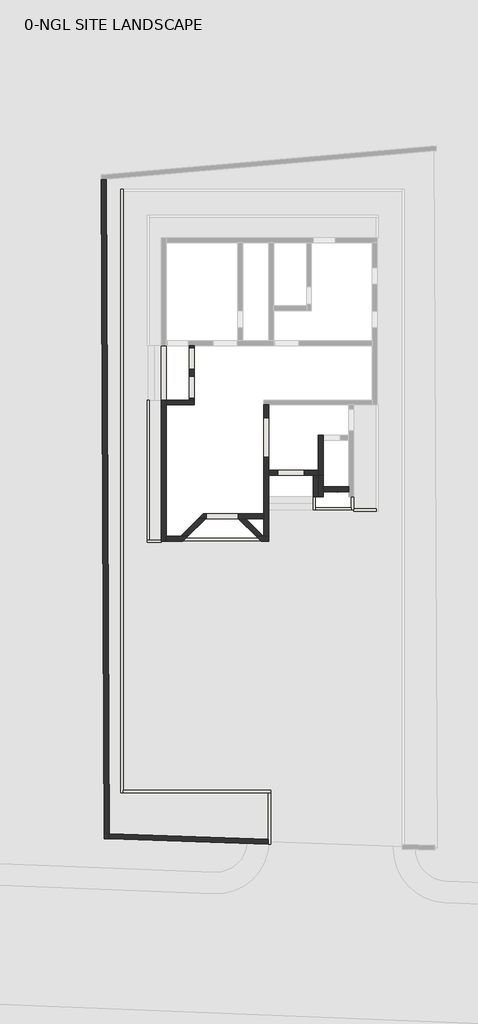
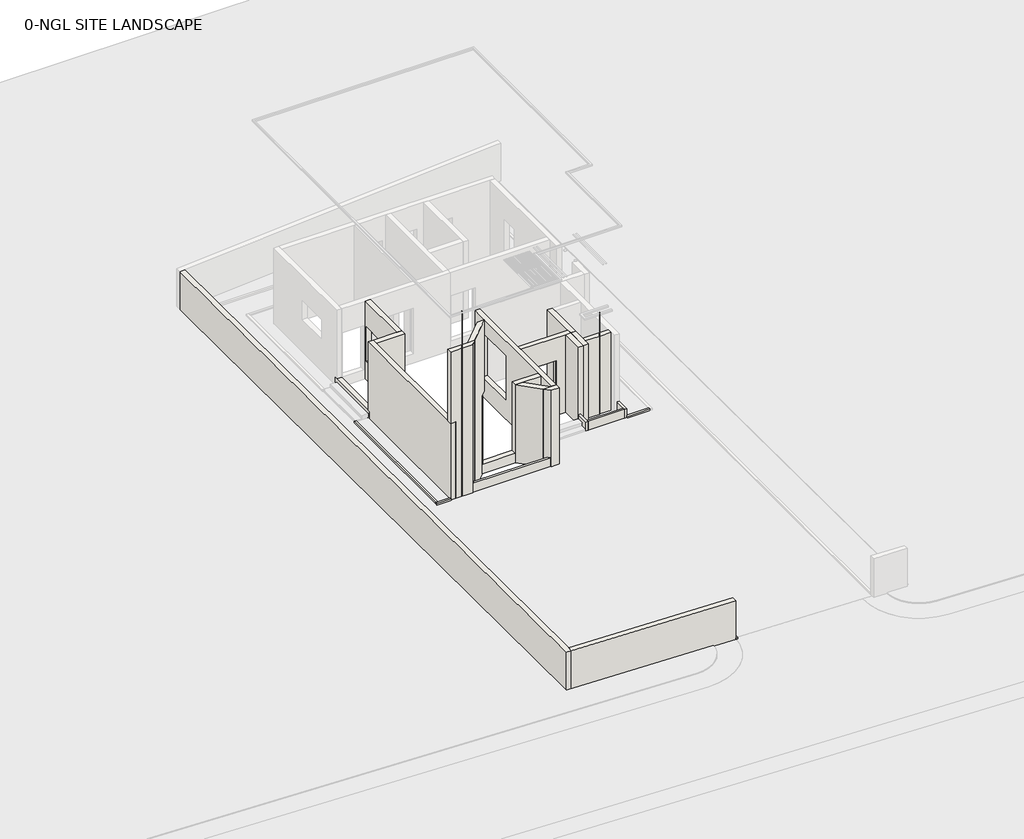
# One storey, part 1 of 2: 27 walls, 2 proxies.
"""IFC4 building model written with IfcOpenShell, lengths in millimetres."""

from ifc_helpers import new_model, si_unit, point, frame, frame_2d, origin, origin_with_axes, place, context, project, spatial, polyline, circle_curve, trimmed, segment, composite_curve, outline, extrude, faceted_brep, element, save
from ifc_brep_helpers import plane_surface, revolved_surface, advanced_brep

model = new_model("IFC4")

# Units and contexts
model_context = context("Model", 3, world=origin())
ifc_project = project(units=[si_unit("LENGTHUNIT", "METRE", prefix="MILLI")], contexts=[model_context])

# Site, building, storey
site = spatial("IfcSite", under=ifc_project)
building = spatial("IfcBuilding", under=site)
storey = spatial("IfcBuildingStorey", under=building, Name="0-NGL SITE LANDSCAPE", Elevation=0.0)

# Proxies
placement = place(None, origin())
element("IfcBuildingElementProxy", 1, Name="Reveal", ObjectType="Reveal", at=placement, inside=storey, context=model_context, shape_type="SweptSolid", body=[
    extrude(outline(composite_curve([segment(trimmed(circle_curve(frame_2d((-9788.8712297, -10317.0014262)), 7.5), [point((-9788.8712297, -10324.5014262))], [point((-9788.8712297, -10309.5014262))], False, "CARTESIAN"), True, "CONTINUOUS"), segment(trimmed(circle_curve(frame_2d((-9788.8712297, -10317.0014262)), 7.5), [point((-9788.8712297, -10309.5014262))], [point((-9788.8712297, -10324.5014262))], False, "CARTESIAN"), True, "CONTINUOUS")], self_intersect=False)), origin_with_axes(), (0.0, 0.0, 1.0), 9000.0),
])
element("IfcBuildingElementProxy", 2, Name="Reveal", ObjectType="Reveal", at=placement, inside=storey, context=model_context, shape_type="SweptSolid", body=[
    extrude(outline(composite_curve([segment(trimmed(circle_curve(frame_2d((-2198.8712297, -8047.0014262)), 7.5), [point((-2198.8712297, -8054.5014262))], [point((-2198.8712297, -8039.5014262))], False, "CARTESIAN"), True, "CONTINUOUS"), segment(trimmed(circle_curve(frame_2d((-2198.8712297, -8047.0014262)), 7.5), [point((-2198.8712297, -8039.5014262))], [point((-2198.8712297, -8054.5014262))], False, "CARTESIAN"), True, "CONTINUOUS")], self_intersect=False)), origin_with_axes(), (0.0, 0.0, 1.0), 3750.0),
    extrude(outline(composite_curve([segment(trimmed(circle_curve(frame_2d((-2198.8712297, -8047.0014262)), 7.5), [point((-2198.8712297, -8054.5014262))], [point((-2198.8712297, -8039.5014262))], False, "CARTESIAN"), True, "CONTINUOUS"), segment(trimmed(circle_curve(frame_2d((-2198.8712297, -8047.0014262)), 7.5), [point((-2198.8712297, -8039.5014262))], [point((-2198.8712297, -8054.5014262))], False, "CARTESIAN"), True, "CONTINUOUS")], self_intersect=False)), frame((0.0, 0.0, 3750.0), z_axis=(0.0, 0.0, 1.0), x_axis=(1.0, 0.0, 0.0)), (0.0, 0.0, 1.0), 1150.0),
])

# Walls
element("IfcWall", 3, ObjectType="100", at=placement, inside=storey, context=model_context, shape_type="Brep", body=[
    faceted_brep([(-3308.8712297, -8277.0014262, 0.0), (-3308.8712297, -8877.0014262, 0.0), (-3308.8712297, -8877.0014262, 500.0), (-3308.8712297, -8277.0014262, 500.0), (-3208.8712297, -8277.0014262, 0.0), (-3208.8712297, -8277.0014262, 500.0), (-3208.8712297, -8777.0014262, 500.0), (-3208.8712297, -8877.0014262, 500.0), (-3208.8712297, -8877.0014262, 0.0), (-3208.8712297, -8777.0014262, 0.0)], [[[0, 1, 2, 3]], [[4, 5, 6, 7, 8, 9]], [[1, 0, 4, 9, 8]], [[3, 2, 7, 6, 5]], [[0, 3, 5, 4]], [[2, 1, 8, 7]]]),
])
element("IfcWall", 4, ObjectType="100", at=placement, inside=storey, context=model_context, shape_type="SweptSolid", body=[
    extrude(outline(polyline([(-1548.8712297, -8877.0014262), (-3208.8712297, -8877.0014262), (-3208.8712297, -8777.0014262), (-1548.8712297, -8777.0014262), (-1548.8712297, -8877.0014262)])), origin_with_axes(), (0.0, 0.0, 1.0), 500.0),
])
element("IfcWall", 5, ObjectType="100", at=placement, inside=storey, context=model_context, shape_type="Brep", body=[
    faceted_brep([(-1448.8712297, -8877.0014262, 500.0), (-1448.8712297, -8877.0014262, 0.0), (-1448.8712297, -8827.0014262, 0.0), (-1448.8712297, -8277.0014262, 0.0), (-1448.8712297, -8277.0014262, 500.0), (-1548.8712297, -8877.0014262, 0.0), (-1548.8712297, -8877.0014262, 500.0), (-1548.8712297, -8777.0014262, 500.0), (-1548.8712297, -8277.0014262, 500.0), (-1548.8712297, -8277.0014262, 0.0), (-1548.8712297, -8777.0014262, 0.0)], [[[0, 1, 2, 3, 4]], [[5, 6, 7, 8, 9, 10]], [[3, 2, 1, 5, 10, 9]], [[4, 3, 9, 8]], [[0, 4, 8, 7, 6]], [[0, 6, 5, 1]]]),
])
element("IfcWall", 6, ObjectType="100", at=placement, inside=storey, context=model_context, shape_type="SweptSolid", body=[
    extrude(outline(polyline([(-5736.5057893, -10292.0014262), (-9283.1448516, -10292.0014262), (-9183.1448516, -10192.0014262), (-5836.5057893, -10192.0014262), (-5736.5057893, -10292.0014262)])), origin_with_axes(), (0.0, 0.0, 1.0), 500.0),
])
element("IfcWall", 7, ObjectType="100", at=placement, inside=storey, context=model_context, shape_type="Brep", body=[
    faceted_brep([(-408.8712297, -8827.0014262, 0.0), (-1448.8712297, -8827.0014262, 0.0), (-1448.8712297, -8827.0014262, 150.0), (-408.8712297, -8827.0014262, 150.0), (-408.8712297, -8927.0014262, 0.0), (-408.8712297, -8927.0014262, 150.0), (-1448.8712297, -8927.0014262, 150.0), (-1448.8712297, -8927.0014262, 0.0), (-1448.8712297, -8877.0014262, 0.0)], [[[0, 1, 2, 3]], [[4, 5, 6, 7]], [[1, 0, 4, 7, 8]], [[3, 2, 6, 5]], [[2, 1, 8, 7, 6]], [[0, 3, 5, 4]]]),
])
element("IfcWall", 8, ObjectType="100", at=placement, inside=storey, context=model_context, shape_type="Brep", body=[
    faceted_brep([(-10958.8712297, -10367.0014262, 0.0), (-10308.8712297, -10367.0014262, 0.0), (-10308.8712297, -10367.0014262, 150.0), (-10958.8712297, -10367.0014262, 150.0), (-10958.8712297, -10267.0014262, 0.0), (-10958.8712297, -10267.0014262, 150.0), (-10858.8712297, -10267.0014262, 150.0), (-10308.8712297, -10267.0014262, 150.0), (-10308.8712297, -10267.0014262, 0.0), (-10858.8712297, -10267.0014262, 0.0), (-10308.8712297, -10317.0014262, 0.0)], [[[0, 1, 2, 3]], [[4, 5, 6, 7, 8, 9]], [[1, 0, 4, 9, 8, 10]], [[3, 2, 7, 6, 5]], [[2, 1, 10, 8, 7]], [[0, 3, 5, 4]]]),
])
element("IfcWall", 9, ObjectType="100", at=placement, inside=storey, context=model_context, shape_type="SweptSolid", body=[
    extrude(outline(polyline([(-10958.8712297, -10267.0014262), (-10958.8712297, -3817.0014262), (-10858.8712297, -3817.0014262), (-10858.8712297, -10267.0014262), (-10958.8712297, -10267.0014262)])), origin_with_axes(), (0.0, 0.0, 1.0), 150.0),
])
element("IfcWall", 10, ObjectType="100", at=placement, inside=storey, context=model_context, shape_type="Brep", body=[
    faceted_brep([(-12158.8712297, 5892.9985738, 0.0), (-12158.8712297, -21892.3863739, 0.0), (-12158.8712297, -21892.3863739, 150.0), (-12158.8712297, 5892.9985738, 150.0), (-12058.8712297, 5892.9985738, 0.0), (-12058.8712297, 5892.9985738, 150.0), (-12058.8712297, 5792.9985738, 150.0), (-12058.8712297, -21792.3863739, 150.0), (-12058.8712297, -21892.3863739, 150.0), (-12058.8712297, -21892.3863739, 0.0), (-12058.8712297, -21792.3863739, 0.0), (-12058.8712297, 5792.9985738, 0.0)], [[[0, 1, 2, 3]], [[4, 5, 6, 7, 8, 9, 10, 11]], [[1, 0, 4, 11, 10, 9]], [[3, 2, 8, 7, 6, 5]], [[2, 1, 9, 8]], [[0, 3, 5, 4]]]),
])
element("IfcWall", 11, ObjectType="100", at=placement, inside=storey, context=model_context, shape_type="Brep", body=[
    faceted_brep([(-12058.8712297, -21892.3863739, 0.0), (-5373.4846863, -21892.3863739, 0.0), (-5273.4846863, -21892.3863739, 0.0), (-5273.4846863, -21892.3863739, 150.0), (-5373.4846863, -21892.3863739, 150.0), (-12058.8712297, -21892.3863739, 150.0), (-12058.8712297, -21792.3863739, 0.0), (-12058.8712297, -21792.3863739, 150.0), (-5273.4846863, -21792.3863739, 150.0), (-5273.4846863, -21792.3863739, 0.0)], [[[0, 1, 2, 3, 4, 5]], [[6, 7, 8, 9]], [[2, 1, 0, 6, 9]], [[5, 4, 3, 8, 7]], [[0, 5, 7, 6]], [[3, 2, 9, 8]]]),
])
element("IfcWall", 12, ObjectType="100", at=placement, inside=storey, context=model_context, shape_type="Brep", body=[
    faceted_brep([(-5373.4846863, -21892.3863739, 0.0), (-5373.4846863, -24043.4760733, 0.0), (-5373.4846863, -24273.6234256, 0.0), (-5373.4846863, -24273.6234256, 150.0), (-5373.4846863, -21892.3863739, 150.0), (-5273.4846863, -21892.3863739, 0.0), (-5273.4846863, -21892.3863739, 150.0), (-5273.4846863, -24277.2035581, 150.0), (-5273.4846863, -24277.2035581, 0.0)], [[[0, 1, 2, 3, 4]], [[5, 6, 7, 8]], [[2, 1, 0, 5, 8]], [[4, 3, 7, 6]], [[0, 4, 6, 5]], [[3, 2, 8, 7]]]),
])
element("IfcWall", 13, ObjectType="230", at=placement, inside=storey, context=model_context, shape_type="Brep", body=[
    faceted_brep([(-5348.8712297, -10087.0014262, 0.0), (-5348.8712297, -7277.0014262, 0.0), (-5348.8712297, -7047.0014262, 0.0), (-5348.8712297, -4047.0014262, 0.0), (-5348.8712297, -4047.0014262, 3750.0), (-5348.8712297, -7047.0014262, 3750.0), (-5348.8712297, -7277.0014262, 3750.0), (-5348.8712297, -10087.0014262, 3750.0), (-5348.8712297, -4632.0061137, 3033.996875), (-5348.8712297, -4632.0061137, 900.0), (-5348.8712297, -6461.9967387, 900.0), (-5348.8712297, -6461.9967387, 3033.996875), (-5578.8712297, -10087.0014262, 0.0), (-5578.8712297, -10087.0014262, 3750.0), (-5578.8712297, -9277.0014262, 3750.0), (-5578.8712297, -9047.0014262, 3750.0), (-5578.8712297, -4047.0014262, 3750.0), (-5578.8712297, -4047.0014262, 0.0), (-5578.8712297, -9047.0014262, 0.0), (-5578.8712297, -9277.0014262, 0.0), (-5578.8712297, -4632.0061137, 3033.996875), (-5578.8712297, -6461.9967387, 3033.996875), (-5578.8712297, -6461.9967387, 900.0), (-5578.8712297, -4632.0061137, 900.0)], [[[0, 1, 2, 3, 4, 5, 6, 7], [8, 9, 10, 11]], [[12, 13, 14, 15, 16, 17, 18, 19], [20, 21, 22, 23]], [[3, 2, 1, 0, 12, 19, 18, 17]], [[7, 6, 5, 4, 16, 15, 14, 13]], [[4, 3, 17, 16]], [[0, 7, 13, 12]], [[9, 8, 20, 23]], [[10, 9, 23, 22]], [[11, 10, 22, 21]], [[8, 11, 21, 20]]]),
])
element("IfcWall", 14, ObjectType="230", at=placement, inside=storey, context=model_context, shape_type="Brep", body=[
    faceted_brep([(-5348.8712297, -7277.0014262, 0.0), (-3308.8712297, -7277.0014262, 0.0), (-3078.8712297, -7277.0014262, 0.0), (-3078.8712297, -7277.0014262, 3750.0), (-3308.8712297, -7277.0014262, 3750.0), (-5348.8712297, -7277.0014262, 3750.0), (-4931.1212297, -7277.0014262, 2639.5), (-3726.6212297, -7277.0014262, 2639.5), (-3726.6212297, -7277.0014262, 450.0), (-4931.1212297, -7277.0014262, 450.0), (-3078.8712297, -7047.0014262, 0.0), (-5348.8712297, -7047.0014262, 0.0), (-5348.8712297, -7047.0014262, 3750.0), (-3078.8712297, -7047.0014262, 3750.0), (-3726.6212297, -7047.0014262, 2639.5), (-4931.1212297, -7047.0014262, 2639.5), (-4931.1212297, -7047.0014262, 450.0), (-3726.6212297, -7047.0014262, 450.0), (-4931.1212297, -7257.0014262, 2639.5), (-3726.6212297, -7257.0014262, 2639.5), (-3726.6212297, -7180.0014262, 2639.5), (-4931.1212297, -7180.0014262, 2639.5), (-4931.1212297, -7257.0014262, 450.0), (-4931.1212297, -7180.0014262, 450.0), (-3726.6212297, -7257.0014262, 450.0), (-3711.6212297, -7257.0014262, 450.0), (-3711.6212297, -7180.0014262, 450.0), (-3726.6212297, -7180.0014262, 450.0), (-4946.1212297, -7180.0014262, 450.0), (-4946.1212297, -7257.0014262, 450.0), (-3711.6212297, -7257.0014262, 2654.5), (-4946.1212297, -7257.0014262, 2654.5), (-4946.1212297, -7180.0014262, 2654.5), (-3711.6212297, -7180.0014262, 2654.5)], [[[0, 1, 2, 3, 4, 5], [6, 7, 8, 9]], [[10, 11, 12, 13], [14, 15, 16, 17]], [[2, 1, 0, 11, 10]], [[5, 4, 3, 13, 12]], [[0, 5, 12, 11]], [[3, 2, 10, 13]], [[6, 18, 19, 7]], [[14, 20, 21, 15]], [[18, 6, 9, 22]], [[15, 21, 23, 16]], [[22, 9, 8, 24, 25, 26, 27, 17, 16, 23, 28, 29]], [[7, 19, 24, 8]], [[20, 14, 17, 27]], [[30, 31, 32, 33]], [[29, 28, 32, 31]], [[21, 20, 27, 26, 33, 32, 28, 23]], [[26, 25, 30, 33]], [[19, 18, 22, 29, 31, 30, 25, 24]]]),
])
element("IfcWall", 15, ObjectType="230", at=placement, inside=storey, context=model_context, shape_type="AdvancedBrep", body=[
    advanced_brep(
    [(-9308.1448516, -10317.0014262, 0.0), (-9308.1448516, -10317.0014262, 7200.0), (-9781.3712297, -10317.0014262, 7200.0), (-9781.3712297, -10317.0014262, 0.0), (-10308.8712297, -10317.0014262, 3750.0), (-10078.8712297, -10317.0014262, 3750.0), (-10078.8712297, -10317.0014262, 0.0), (-9796.3712297, -10317.0014262, 0.0), (-9796.3712297, -10317.0014262, 7200.0), (-10308.8712297, -10317.0014262, 7200.0), (-9078.1448516, -10087.0014262, 0.0), (-9403.4139709, -10087.0014262, 0.0), (-10078.8712297, -10087.0014262, 0.0), (-10078.8712297, -10087.0014262, 3750.0), (-10308.8712297, -10087.0014262, 3750.0), (-10308.8712297, -10087.0014262, 7200.0), (-10078.8712297, -10087.0014262, 7200.0), (-9403.4139709, -10087.0014262, 7200.0), (-9078.1448516, -10087.0014262, 7200.0), (-9183.1448516, -10192.0014262, 0.0), (-9283.1448516, -10292.0014262, 0.0), (-9788.8712297, -10309.5014262, 0.0), (-9788.8712297, -10309.5014262, 7200.0)],
    [
        (0, 1),
        (1, 2),
        (2, 3),
        (3, 0),
        (4, 5),
        (5, 6),
        (6, 7),
        (7, 8),
        (8, 9),
        (9, 4),
        (10, 11),
        (11, 12),
        (12, 13),
        (13, 14),
        (14, 15),
        (15, 16),
        (16, 17),
        (17, 18),
        (18, 10),
        (10, 19),
        (19, 20),
        (20, 0),
        (3, 21, circle_curve(frame((-9788.8712297, -10317.0014262, 0.0), z_axis=(0.0, 0.0, 1.0), x_axis=(0.0, 1.0, 0.0)), 7.5)),
        (21, 7, circle_curve(frame((-9788.8712297, -10317.0014262, 0.0), z_axis=(0.0, 0.0, 1.0), x_axis=(0.0, 1.0, 0.0)), 7.5)),
        (6, 12),
        (15, 9),
        (8, 22, circle_curve(frame((-9788.8712297, -10317.0014262, 7200.0), z_axis=(0.0, 0.0, -1.0), x_axis=(0.0, 1.0, 0.0)), 7.5)),
        (22, 2, circle_curve(frame((-9788.8712297, -10317.0014262, 7200.0), z_axis=(0.0, 0.0, -1.0), x_axis=(0.0, 1.0, 0.0)), 7.5)),
        (1, 18),
        (22, 21),
        (13, 5),
        (4, 14),
    ],
    [
        plane_surface(frame((-10193.8712297, -10317.0014262, 0.0), z_axis=(0.0, -1.0, 0.0), x_axis=(1.0, 0.0, 0.0))),
        plane_surface(frame((-10193.8712297, -10087.0014262, 0.0), z_axis=(0.0, 1.0, 0.0), x_axis=(-1.0, 0.0, 0.0))),
        plane_surface(frame((-10193.8712297, -10317.0014262, 0.0), z_axis=(0.0, 0.0, -1.0), x_axis=(0.0, 1.0, 0.0))),
        plane_surface(frame((-9355.7794112, -10317.0014262, 7200.0), z_axis=(0.0, 0.0, 1.0), x_axis=(0.0, 1.0, 0.0))),
        revolved_surface(polyline([(-9788.8712297, -10309.5014262, 7200.0), (-9788.8712297, -10309.5014262, 0.0)]), (-9788.8712297, -10317.0014262, 9000.0), (0.0, 0.0, 1.0)),
        plane_surface(frame((-10193.8712297, -10317.0014262, 3750.0), z_axis=(0.0, 0.0, -1.0), x_axis=(1.0, 0.0, 0.0))),
        plane_surface(frame((-10078.8712297, -2762.0014262, 0.0), z_axis=(-1.0, 0.0, 0.0), x_axis=(0.0, 1.0, 0.0))),
        plane_surface(frame((-10308.8712297, -10162.0014262, 3750.0), z_axis=(-1.0, 0.0, 0.0), x_axis=(0.0, -1.0, 0.0))),
        plane_surface(frame((-8866.2081314, -9875.064706, 0.0), z_axis=(0.7071067811865475, -0.7071067811865477, 0.0), x_axis=(0.7071067811865477, 0.7071067811865475, 0.0))),
    ],
    [
        (0, [[1, 2, 3, 4]]),
        (0, [[5, 6, 7, 8, 9, 10]]),
        (1, [[11, 12, 13, 14, 15, 16, 17, 18, 19]]),
        (2, [[-12, -11, 20, 21, 22, -4, 23, 24, -7, 25]]),
        (3, [[-18, -17, -16, 26, -9, 27, 28, -2, 29]]),
        (4, [[30, -23, -3, -28]]),
        (4, [[-30, -27, -8, -24]]),
        (5, [[-14, 31, -5, 32]]),
        (6, [[-25, -6, -31, -13]]),
        (7, [[-26, -15, -32, -10]]),
        (8, [[-22, -21, -20, -19, -29, -1]]),
    ],
),
])
element("IfcWall", 16, ObjectType="230", at=placement, inside=storey, context=model_context, shape_type="Brep", body=[
    faceted_brep([(-9078.1448516, -10087.0014262, 7200.0), (-9078.1448516, -10087.0014262, 0.0), (-8268.1448516, -9277.0014262, 0.0), (-8268.1448516, -9277.0014262, 3750.0), (-8243.8712297, -9252.7278043, 3750.0), (-8038.1448516, -9047.0014262, 3750.0), (-8038.1448516, -9047.0014262, 7200.0), (-8243.8712297, -9252.7278043, 7200.0), (-8268.1448516, -9277.0014262, 7200.0), (-9403.4139709, -10087.0014262, 0.0), (-9403.4139709, -10087.0014262, 7200.0), (-8363.4139709, -9047.0014262, 7200.0), (-8363.4139709, -9047.0014262, 3750.0), (-8593.4139709, -9277.0014262, 3750.0), (-8593.4139709, -9277.0014262, 0.0), (-8243.8712297, -9047.0014262, 3750.0)], [[[0, 1, 2, 3, 4, 5, 6, 7, 8]], [[9, 10, 11, 12, 13, 14]], [[2, 1, 9, 14]], [[0, 8, 7, 6, 11, 10]], [[0, 10, 9, 1]], [[12, 15, 5, 4, 3, 13]], [[3, 2, 14, 13]], [[6, 5, 15, 12, 11]]]),
])
element("IfcWall", 17, ObjectType="230", at=placement, inside=storey, context=model_context, shape_type="Brep", body=[
    faceted_brep([(-8593.4139709, -9277.0014262, 0.0), (-8268.1448516, -9277.0014262, 0.0), (-6751.5057893, -9277.0014262, 0.0), (-6426.23667, -9277.0014262, 0.0), (-5578.8712297, -9277.0014262, 0.0), (-5578.8712297, -9277.0014262, 3750.0), (-6426.23667, -9277.0014262, 3750.0), (-6751.5057893, -9277.0014262, 3750.0), (-6763.8712297, -9277.0014262, 3750.0), (-6763.8712297, -9277.0014262, 450.0), (-8243.8712297, -9277.0014262, 450.0), (-8243.8712297, -9277.0014262, 3750.0), (-8268.1448516, -9277.0014262, 3750.0), (-8593.4139709, -9277.0014262, 3750.0), (-5578.8712297, -9047.0014262, 0.0), (-8363.4139709, -9047.0014262, 0.0), (-8363.4139709, -9047.0014262, 3750.0), (-8243.8712297, -9047.0014262, 3750.0), (-8243.8712297, -9047.0014262, 450.0), (-6763.8712297, -9047.0014262, 450.0), (-6763.8712297, -9047.0014262, 3750.0), (-5578.8712297, -9047.0014262, 3750.0)], [[[0, 1, 2, 3, 4, 5, 6, 7, 8, 9, 10, 11, 12, 13]], [[14, 15, 16, 17, 18, 19, 20, 21]], [[4, 3, 2, 1, 0, 15, 14]], [[5, 21, 20, 8, 7, 6]], [[16, 13, 12, 11, 17]], [[5, 4, 14, 21]], [[10, 18, 17, 11]], [[19, 9, 8, 20]], [[18, 10, 9, 19]], [[0, 13, 16, 15]]]),
])
element("IfcWall", 18, ObjectType="230", at=placement, inside=storey, context=model_context, shape_type="Brep", body=[
    faceted_brep([(-5348.8712297, -10087.0014262, 0.0), (-5578.8712297, -10087.0014262, 0.0), (-5616.23667, -10087.0014262, 0.0), (-5941.5057893, -10087.0014262, 0.0), (-5941.5057893, -10087.0014262, 3750.0), (-5616.23667, -10087.0014262, 3750.0), (-5578.8712297, -10087.0014262, 3750.0), (-5348.8712297, -10087.0014262, 3750.0), (-5348.8712297, -10317.0014262, 0.0), (-5348.8712297, -10317.0014262, 3750.0), (-5711.5057893, -10317.0014262, 3750.0), (-5711.5057893, -10317.0014262, 0.0), (-5736.5057893, -10292.0014262, 0.0), (-5836.5057893, -10192.0014262, 0.0)], [[[0, 1, 2, 3, 4, 5, 6, 7]], [[8, 9, 10, 11]], [[3, 2, 1, 0, 8, 11, 12, 13]], [[7, 6, 5, 4, 10, 9]], [[0, 7, 9, 8]], [[3, 13, 12, 11, 10, 4]]]),
])
element("IfcWall", 19, ObjectType="230", at=placement, inside=storey, context=model_context, shape_type="SweptSolid", body=[
    extrude(outline(polyline([(-6426.23667, -9277.0014262), (-5616.23667, -10087.0014262), (-5941.5057893, -10087.0014262), (-6751.5057893, -9277.0014262), (-6426.23667, -9277.0014262)])), origin_with_axes(), (0.0, 0.0, 1.0), 3750.0),
])
element("IfcWall", 20, ObjectType="230", at=placement, inside=storey, context=model_context, shape_type="SweptSolid", body=[
    extrude(outline(polyline([(-3817.0014262, 0.0), (-3817.0014262, 3750.0), (-1317.0014262, 3750.0), (-1317.0014262, 0.0), (-3817.0014262, 0.0)]), holes=[polyline([(-2402.0014262, 900.0), (-1402.0014262, 900.0), (-1402.0014262, 2550.0), (-2402.0014262, 2550.0), (-2402.0014262, 900.0)]), polyline([(-3732.0014262, 900.0), (-2732.0014262, 900.0), (-2732.0014262, 2550.0), (-3732.0014262, 2550.0), (-3732.0014262, 900.0)])]), frame((-9008.8712297, 0.0, 0.0), z_axis=(1.0, 0.0, 0.0), x_axis=(0.0, 1.0, 0.0)), (0.0, 0.0, 1.0), 230.0),
])
element("IfcWall", 21, ObjectType="230", at=placement, inside=storey, context=model_context, shape_type="Brep", body=[
    faceted_brep([(-3078.8712297, -5432.0014262, 0.0), (-3078.8712297, -7047.0014262, 0.0), (-3078.8712297, -7277.0014262, 0.0), (-3078.8712297, -7277.0014262, 3750.0), (-3078.8712297, -7047.0014262, 3750.0), (-3078.8712297, -5432.0014262, 3750.0), (-2848.8712297, -7277.0014262, 0.0), (-2848.8712297, -5662.0014262, 0.0), (-2848.8712297, -5432.0014262, 0.0), (-2848.8712297, -5432.0014262, 450.0), (-2848.8712297, -5662.0014262, 450.0), (-2848.8712297, -5662.0014262, 2575.0), (-2848.8712297, -5432.0014262, 2575.0), (-2848.8712297, -5432.0014262, 3750.0), (-2848.8712297, -5662.0014262, 3750.0), (-2848.8712297, -7277.0014262, 3750.0), (-2863.8712297, -5432.0014262, 2575.0), (-2863.8712297, -5432.0014262, 450.0), (-2863.8712297, -5662.0014262, 450.0), (-2863.8712297, -5662.0014262, 2575.0)], [[[0, 1, 2, 3, 4, 5]], [[6, 7, 8, 9, 10, 11, 12, 13, 14, 15]], [[2, 1, 0, 8, 7, 6]], [[5, 4, 3, 15, 14, 13]], [[3, 2, 6, 15]], [[0, 5, 13, 12, 16, 17, 9, 8]], [[18, 19, 11, 10]], [[19, 18, 17, 16]], [[19, 16, 12, 11]], [[17, 18, 10, 9]]]),
])
element("IfcWall", 22, ObjectType="230", at=placement, inside=storey, context=model_context, shape_type="Brep", body=[
    faceted_brep([(-3078.8712297, -7277.0014262, 0.0), (-3078.8712297, -8277.0014262, 0.0), (-3078.8712297, -8277.0014262, 3750.0), (-3078.8712297, -7277.0014262, 3750.0), (-2848.8712297, -7277.0014262, 0.0), (-2848.8712297, -7277.0014262, 3750.0), (-2848.8712297, -7817.0014262, 3750.0), (-2848.8712297, -8047.0014262, 3750.0), (-2848.8712297, -8277.0014262, 3750.0), (-2848.8712297, -8277.0014262, 0.0), (-2848.8712297, -8047.0014262, 0.0), (-2848.8712297, -7817.0014262, 0.0)], [[[0, 1, 2, 3]], [[4, 5, 6, 7, 8, 9, 10, 11]], [[1, 0, 4, 11, 10, 9]], [[2, 1, 9, 8]], [[3, 2, 8, 7, 6, 5]], [[0, 3, 5, 4]]]),
])
element("IfcWall", 23, ObjectType="230", at=placement, inside=storey, context=model_context, shape_type="Brep", body=[
    faceted_brep([(-3308.8712297, -7277.0014262, 0.0), (-3308.8712297, -8277.0014262, 0.0), (-3308.8712297, -8277.0014262, 500.0), (-3308.8712297, -8277.0014262, 3750.0), (-3308.8712297, -7277.0014262, 3750.0), (-3078.8712297, -7277.0014262, 0.0), (-3078.8712297, -7277.0014262, 3750.0), (-3078.8712297, -8277.0014262, 3750.0), (-3078.8712297, -8277.0014262, 0.0), (-3208.8712297, -8277.0014262, 0.0)], [[[0, 1, 2, 3, 4]], [[5, 6, 7, 8]], [[1, 0, 5, 8, 9]], [[3, 2, 1, 9, 8, 7]], [[4, 3, 7, 6]], [[0, 4, 6, 5]]]),
])
element("IfcWall", 24, ObjectType="230", at=placement, inside=storey, context=model_context, shape_type="SweptSolid", body=[
    extrude(outline(composite_curve([segment(polyline([(-2848.8712297, -7817.0014262), (-1678.8712297, -7817.0014262), (-1678.8712297, -8047.0014262), (-2191.3712297, -8047.0014262)]), True, "CONTINUOUS"), segment(trimmed(circle_curve(frame_2d((-2198.8712297, -8047.0014262)), 7.5), [point((-2191.3712297, -8047.0014262))], [point((-2198.8712297, -8039.5014262))], True, "CARTESIAN"), True, "CONTINUOUS"), segment(trimmed(circle_curve(frame_2d((-2198.8712297, -8047.0014262)), 7.5), [point((-2198.8712297, -8039.5014262))], [point((-2206.3712297, -8047.0014262))], True, "CARTESIAN"), True, "CONTINUOUS"), segment(polyline([(-2206.3712297, -8047.0014262), (-2848.8712297, -8047.0014262), (-2848.8712297, -7817.0014262)]), True, "CONTINUOUS")], self_intersect=False)), origin_with_axes(), (0.0, 0.0, 1.0), 3750.0),
])
element("IfcWall", 25, ObjectType="230", at=placement, inside=storey, context=model_context, shape_type="Brep", body=[
    faceted_brep([(-8778.8712297, -3817.0014262, 0.0), (-9008.8712297, -3817.0014262, 0.0), (-10078.8712297, -3817.0014262, 0.0), (-10078.8712297, -3817.0014262, 450.0), (-10078.8712297, -3817.0014262, 3750.0), (-9008.8712297, -3817.0014262, 3750.0), (-8778.8712297, -3817.0014262, 3750.0), (-8778.8712297, -4047.0014262, 0.0), (-8778.8712297, -4047.0014262, 3750.0), (-10078.8712297, -4047.0014262, 3750.0), (-10078.8712297, -4047.0014262, 0.0), (-10078.8712297, -3932.0014262, 0.0)], [[[0, 1, 2, 3, 4, 5, 6]], [[7, 8, 9, 10]], [[2, 1, 0, 7, 10, 11]], [[6, 5, 4, 9, 8]], [[0, 6, 8, 7]], [[2, 11, 10, 9, 4, 3]]]),
])
element("IfcWall", 26, ObjectType="230", at=placement, inside=storey, context=model_context, shape_type="Brep", body=[
    faceted_brep([(-10308.8712297, -1202.0014262, 0.0), (-10308.8712297, -3932.0014262, 0.0), (-10308.8712297, -3932.0014262, 450.0), (-10308.8712297, -1202.0014262, 450.0), (-10078.8712297, -1202.0014262, 0.0), (-10078.8712297, -1202.0014262, 450.0), (-10078.8712297, -1317.0014262, 450.0), (-10078.8712297, -3817.0014262, 450.0), (-10078.8712297, -3932.0014262, 450.0), (-10078.8712297, -3932.0014262, 0.0), (-10078.8712297, -3817.0014262, 0.0), (-10078.8712297, -1317.0014262, 0.0)], [[[0, 1, 2, 3]], [[4, 5, 6, 7, 8, 9, 10, 11]], [[1, 0, 4, 11, 10, 9]], [[2, 1, 9, 8]], [[3, 2, 8, 7, 6, 5]], [[0, 3, 5, 4]]]),
])
element("IfcWall", 27, ObjectType="230", at=placement, inside=storey, context=model_context, shape_type="Brep", body=[
    faceted_brep([(-10308.8712297, -3932.0014262, 0.0), (-10308.8712297, -10267.0014262, 0.0), (-10308.8712297, -10317.0014262, 0.0), (-10308.8712297, -10317.0014262, 3750.0), (-10308.8712297, -10087.0014262, 3750.0), (-10308.8712297, -3817.0014262, 3750.0), (-10308.8712297, -3817.0014262, 450.0), (-10308.8712297, -3932.0014262, 450.0), (-10078.8712297, -3932.0014262, 0.0), (-10078.8712297, -3932.0014262, 450.0), (-10078.8712297, -3817.0014262, 450.0), (-10078.8712297, -3817.0014262, 3750.0), (-10078.8712297, -4047.0014262, 3750.0), (-10078.8712297, -10087.0014262, 3750.0), (-10078.8712297, -10317.0014262, 3750.0), (-10078.8712297, -10317.0014262, 0.0), (-10078.8712297, -10087.0014262, 0.0), (-10078.8712297, -4047.0014262, 0.0)], [[[0, 1, 2, 3, 4, 5, 6, 7]], [[8, 9, 10, 11, 12, 13, 14, 15, 16, 17]], [[2, 1, 0, 8, 17, 16, 15]], [[5, 4, 3, 14, 13, 12, 11]], [[0, 7, 9, 8]], [[6, 10, 9, 7]], [[6, 5, 11, 10]], [[2, 15, 14, 3]]]),
])
element("IfcWall", 28, ObjectType="230", at=placement, inside=storey, context=model_context, shape_type="Brep", body=[
    faceted_brep([(-13056.2467144, 6312.39333, 0.0), (-12932.9945123, -24002.9829581, 0.0), (-12932.9945123, -24002.9829581, 1950.0), (-13056.2467144, 6312.39333, 1950.0), (-12826.325768, 6332.305069, 0.0), (-12826.325768, 6332.305069, 1950.0), (-12703.8949668, -23781.037673, 1950.0), (-12702.9591283, -24011.2185296, 1950.0), (-12702.9591283, -24011.2185296, 0.0), (-12703.8949668, -23781.037673, 0.0)], [[[0, 1, 2, 3]], [[4, 5, 6, 7, 8, 9]], [[1, 0, 4, 9, 8]], [[3, 2, 7, 6, 5]], [[0, 3, 5, 4]], [[2, 1, 8, 7]]]),
])
element("IfcWall", 29, ObjectType="230", at=placement, inside=storey, context=model_context, shape_type="Brep", body=[
    faceted_brep([(-12702.9591283, -24011.2185296, 0.0), (-5373.4846863, -24273.6234256, 0.0), (-5373.4846863, -24273.6234256, 150.0), (-5373.4846863, -24273.6234256, 1950.0), (-12702.9591283, -24011.2185296, 1950.0), (-12703.8949668, -23781.037673, 0.0), (-12703.8949668, -23781.037673, 1950.0), (-5373.4846863, -24043.4760733, 1950.0), (-5373.4846863, -24043.4760733, 0.0)], [[[0, 1, 2, 3, 4]], [[5, 6, 7, 8]], [[1, 0, 5, 8]], [[4, 3, 7, 6]], [[0, 4, 6, 5]], [[3, 2, 1, 8, 7]]]),
])

save(model, "model.ifc")

# Revit data of these elements
# Type "100"
#   Layers, outside or top first: 100 mm "Default Wall" (function 1)
# Type "230"
#   Layers, outside or top first: 230 mm "Default Wall" (function 1)
# Elements 3, 4, 5, 6 (IfcWall, "100")
#   Top Offset = 50 mm
#   Base Offset = 0 mm
#   wall height = 500 mm
#   Phase Created = New Construction
#   Base Constraint = 0-NGL SITE LANDSCAPE
#   Top Constraint = 01- GROUND FLOOR
#   Materials on its faces: "Default Wall"
# Elements 7, 8, 9, 10, 11, 12 (IfcWall, "100")
#   Top Offset = 150 mm
#   Base Offset = 0 mm
#   wall height = 150 mm
#   Phase Created = New Construction
#   Base Constraint = 0-NGL SITE LANDSCAPE
#   Top Constraint = 0-NGL SITE LANDSCAPE
#   Materials on its faces: "Default Wall"
# Elements 13, 14, 17, 18, 19, 20, 21, 22, 23, 25, 27 (IfcWall, "230")
#   Top Offset = 0 mm
#   Base Offset = 0 mm
#   wall height = 3750 mm
#   Phase Created = New Construction
#   Base Constraint = 0-NGL SITE LANDSCAPE
#   Top Constraint = S1
#   Materials on its faces: "Default Wall"
# Elements 15, 16 (IfcWall, "230")
#   Top Offset = 0 mm
#   Base Offset = 0 mm
#   wall height = 7200 mm
#   Phase Created = New Construction
#   Base Constraint = 0-NGL SITE LANDSCAPE
#   Top Constraint = S2
#   Materials on its faces: "Default Wall"
# Element 24 (IfcWall, "230")
#   Top Offset = 0 mm
#   Base Offset = 0 mm
#   wall height = 3750 mm
#   Phase Created = New Construction
#   Base Constraint = 0-NGL SITE LANDSCAPE
#   Top Constraint = S1
#   Materials on its faces: "Default Wall", "Brick 04"
# Element 26 (IfcWall, "230")
#   Top Offset = 0 mm
#   Base Offset = 0 mm
#   wall height = 450 mm
#   Phase Created = New Construction
#   Base Constraint = 0-NGL SITE LANDSCAPE
#   Top Constraint = 01- GROUND FLOOR
#   Materials on its faces: "Default Wall", "Marble 06"
# Elements 28, 29 (IfcWall, "230")
#   Top Offset = 1500 mm
#   Base Offset = 0 mm
#   wall height = 1950 mm
#   Phase Created = New Construction
#   Base Constraint = 0-NGL SITE LANDSCAPE
#   Top Constraint = 01- GROUND FLOOR
#   Materials on its faces: "Default Wall"
# Materials
#   "Default Wall": colour RGB 255 255 255, transparency 0, Cost = 0
#   "Brick 04": colour RGB 80 80 80, transparency 0
#   "Marble 06": colour RGB 58 58 58, transparency 0, Cost = 0
